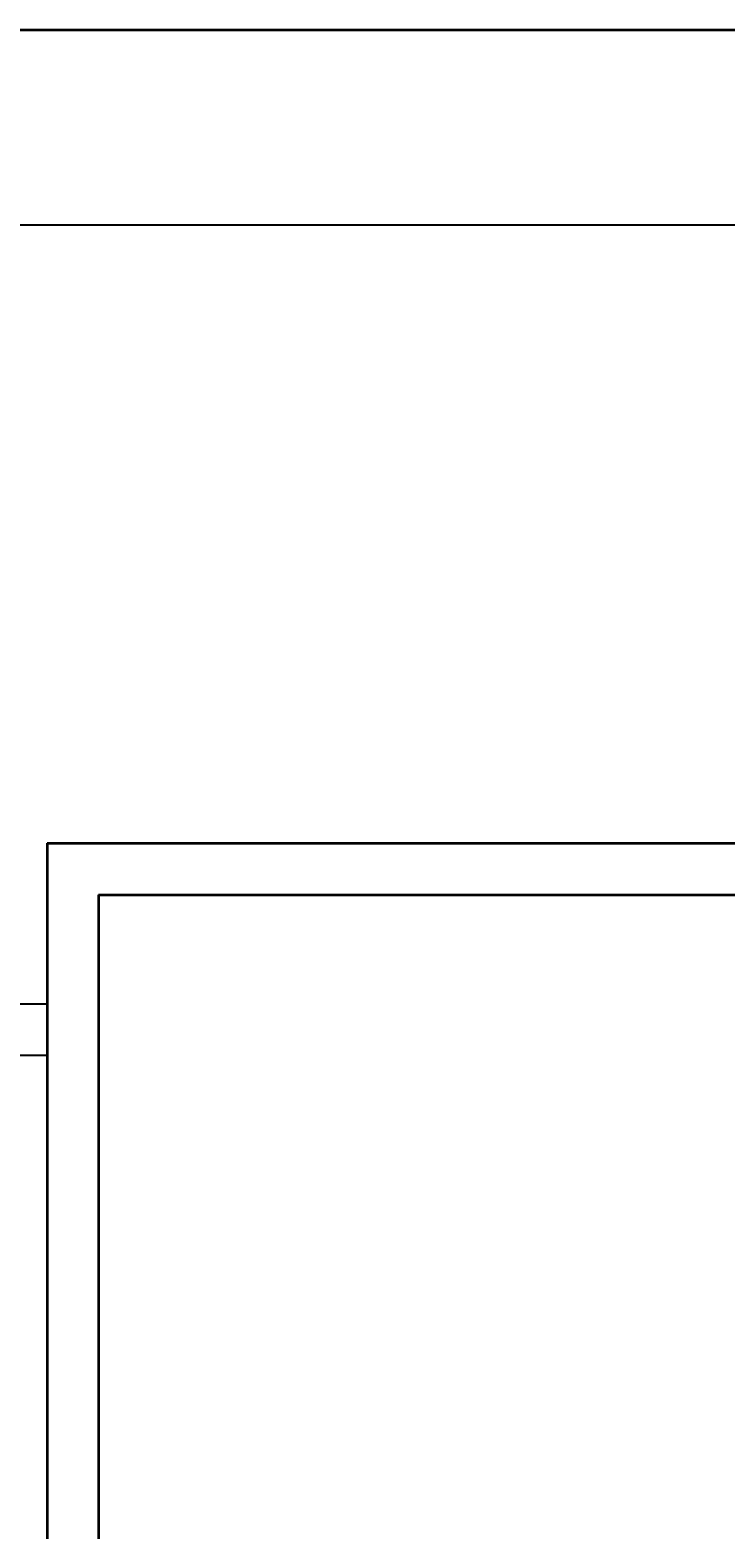
# Model space of a CAD drawing. Units: inches. Extents: x 1088 to 1703, y 668 to 1875.
# Tile 41 of 45: x 1436 to 1497, y 1743 to 1875. Entities that reach past the tile are written whole.
import ezdxf

# ---------------------------------------------------------------- set-up
doc = ezdxf.new("R2010")
doc.units = ezdxf.units.IN
for name, color, linetype, lineweight in [('A-ANNO-DIMS', 2, 'Continuous', 18), ('A-ANNO-TTLB', 7, 'Continuous', 35), ('A-FLOR-HRAL', 7, 'Continuous', 25), ('A-WALL', 7, 'Continuous', 35)]:
    doc.layers.add(name, color=color, linetype=linetype, lineweight=lineweight)
doc.styles.get("Standard").update_dxf_attribs({"font": 'arial.ttf'})
doc.dimstyles.get("Standard").update_dxf_attribs({"dimtxt": 0.18, "dimasz": 0.18, "dimexe": 0.18, "dimexo": 0.0625, "dimgap": 0.09, "dimtad": 0, "dimtih": 1, "dimtoh": 1, "dimdec": 4, "dimzin": 0, "dimdsep": 46, "dimtxsty": 'Standard', "dimcen": 0.09, "dimadec": 0, "dimazin": 0, "dimtfac": 1, "dimtdec": 4, "dimtofl": 0, "dimtmove": 0, "dimatfit": 3, "dimfxl": 1, "dimtolj": 1, "dimtzin": 0, "dimarcsym": 0})

# ---------------------------------------------------------------- blocks, each defined once
blk = doc.blocks.new('*D28')
at = {"layer": 'A-ANNO-DIMS', "color": 0, "lineweight": -2, "transparency": 16777216}
for p, q in [((1170.34, 1803.62), (1170.34, 1857.79)), ((1170.52, 1857.61), (1408.15, 1857.61)), ((1646.56, 1857.61), (1408.94, 1857.61)), ((1646.74, 1745.55), (1646.74, 1857.79))]:
    blk.add_line(p, q, dxfattribs=at)
at = {"layer": 'A-ANNO-DIMS', "color": 0, "transparency": 16777216}
for points in [[(1170.52, 1857.64), (1170.52, 1857.58), (1170.34, 1857.61)], [(1646.56, 1857.64), (1646.56, 1857.58), (1646.74, 1857.61)]]:
    blk.add_solid(points, dxfattribs=at)
at = {"layer": 'Defpoints', "color": 0, "transparency": 16777216}
for p in [(1646.74, 1857.61), (1170.34, 1803.56), (1646.74, 1745.49)]:
    blk.add_point(p, dxfattribs=at)
at = {"layer": 'A-ANNO-DIMS', "color": 0, "transparency": 16777216, "insert": (1408.54, 1857.61), "char_height": 0.18, "attachment_point": 5}
blk.add_mtext('\\A1;476.4', dxfattribs=at)

msp = doc.modelspace()

# ---------------------------------------------------------------- linework, layer by layer
at = {"layer": 'A-ANNO-TTLB'}
msp.add_lwpolyline([(1088.369, 1874.677), (1703.181, 1874.677), (1703.181, 667.947), (1088.369, 667.947)], close=True, dxfattribs=at)
at = {"layer": 'A-FLOR-HRAL'}
for p, q in [((1317.345, 1789.507), (1437.345, 1789.507)), ((1437.345, 1785.007), (1317.345, 1785.007))]:
    msp.add_line(p, q, dxfattribs=at)
at = {"layer": 'A-WALL'}
for p, q in [((1437.345, 1803.558), (1437.345, 1668.558)), ((1437.345, 1803.558), (1624.845, 1803.558)), ((1437.345, 1803.558), (1624.845, 1803.558)), ((1437.345, 1803.558), (1624.845, 1803.558)), ((1437.345, 1803.558), (1624.845, 1803.558)), ((1437.345, 1803.558), (1624.845, 1803.558)), ((1441.845, 1799.058), (1441.845, 1673.058)), ((1441.845, 1799.058), (1620.345, 1799.058)), ((1437.345, 1779.956), (1437.345, 1775.456))]:
    msp.add_line(p, q, dxfattribs=at)

# ---------------------------------------------------------------- dimensions: what is measured, and where the dimension line sits
at = {"layer": 'A-ANNO-DIMS'}
dim = msp.add_linear_dim(base=(1646.743, 1857.608), p1=(1170.345, 1803.558), p2=(1646.743, 1745.49), dimstyle='Standard', override={"dimdec": 1, "dimlfac": 1, "dimrnd": 0, "dimzin": 0, "dimdsep": 46, "dimlunit": 2}, dxfattribs=at)
dim.commit()
dim.dimension.update_dxf_attribs({"geometry": '*D28', "text_midpoint": (1408.544, 1857.608)})

doc.saveas('drawing.dxf')
